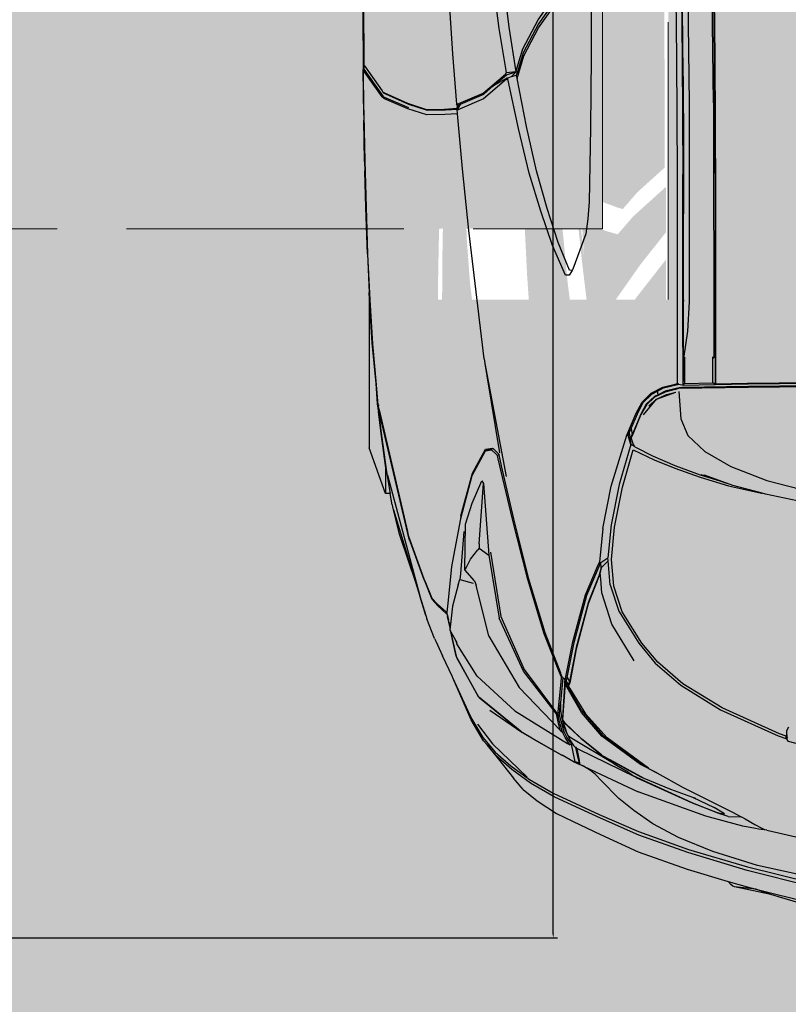
# Model space of a CAD drawing. Units: inches. Extents: x 1884 to 2398, y 474 to 1488.
# Tile 19 of 39: x 2275 to 2308, y 577 to 620. Entities that reach past the tile are written whole.
import ezdxf

# ---------------------------------------------------------------- set-up
doc = ezdxf.new("R2010")
doc.units = ezdxf.units.IN
doc.header["$MEASUREMENT"] = 0
doc.linetypes.add('ACAD_ISO02W100', pattern=[15, 12, -3])
doc.layers.get('0').update_dxf_attribs({"color": 250})
for name, color, linetype, lineweight in [('A-ANNO-DIMS', 2, 'Continuous', 18), ('A-FLOR-OVHD', 8, 'ACAD_ISO02W100', 18), ('C-VEHI', 8, 'Continuous', 18)]:
    doc.layers.add(name, color=color, linetype=linetype, lineweight=lineweight)
doc.layers.add('Edges', color=250, linetype='Continuous')
doc.layers.add('L-PVMT-PATT', color=9, linetype='Continuous', lineweight=13, true_color=0xc7c8ca)
doc.styles.get("Standard").update_dxf_attribs({"font": 'arial.ttf'})
doc.dimstyles.get("Standard").update_dxf_attribs({"dimtxt": 7, "dimasz": 0.18, "dimexe": 0.18, "dimexo": 0.0625, "dimgap": 0.09, "dimtad": 0, "dimtih": 1, "dimtoh": 1, "dimzin": 0, "dimdsep": 46, "dimlunit": 3, "dimtxsty": 'Standard', "dimcen": 0.09, "dimadec": 0, "dimazin": 0, "dimtfac": 1, "dimtofl": 0, "dimtmove": 0, "dimatfit": 3, "dimfxl": 1, "dimtolj": 1, "dimtzin": 0, "dimarcsym": 0})

# ---------------------------------------------------------------- blocks, each defined once
blk = doc.blocks.new('Nissan Qashqai pl')
at = {"layer": 'Edges'}
for p, q in [((11.0572, 11.4499), (11.056, 11.559)), ((11.0579, 11.4504), (11.0566, 11.5593)), ((11.0595, 11.5599), (11.0607, 11.4508)), ((11.0606, 11.5601), (11.0618, 11.4509)), ((11.6016, 11.5276), (11.5866, 11.4607)), ((11.5884, 11.4499), (11.6076, 11.5276)), ((11.6118, 11.5276), (11.5922, 11.4494)), ((11.6127, 11.4589), (11.6297, 11.5276)), ((11.164, 11.4711), (11.1776, 11.5231)), ((11.4503, 11.4945), (11.4568, 11.5197)), ((11.1877, 11.5111), (11.1791, 11.4696)), ((11.5481, 11.471), (11.5571, 11.511)), ((11.6277, 11.5063), (11.6224, 11.4874)), ((11.435, 11.4947), (11.439, 11.4927)), ((11.439, 11.4927), (11.4437, 11.4925)), ((11.4447, 11.4924), (11.4422, 11.4848)), ((11.4451, 11.4934), (11.4432, 11.4935)), ((11.4437, 11.4925), (11.4449, 11.4929)), ((11.4447, 11.4924), (11.4437, 11.4925)), ((11.4445, 11.4833), (11.4478, 11.493)), ((11.4449, 11.4929), (11.4447, 11.4924)), ((11.4462, 11.4924), (11.4447, 11.4924)), ((11.4449, 11.4929), (11.4461, 11.4934)), ((11.4451, 11.4934), (11.4449, 11.4929)), ((11.4461, 11.4934), (11.4451, 11.4934)), ((11.4479, 11.4933), (11.4461, 11.4934)), ((11.4479, 11.4933), (11.4462, 11.4924)), ((11.4478, 11.493), (11.4462, 11.4924)), ((11.4502, 11.4939), (11.4478, 11.493)), ((11.4503, 11.4945), (11.4479, 11.4932)), ((11.4479, 11.4932), (11.4479, 11.4933)), ((11.4502, 11.4939), (11.4503, 11.4945)), ((11.4422, 11.4848), (11.4138, 11.4219)), ((11.4159, 11.42), (11.4445, 11.4833)), ((11.6224, 11.4874), (11.6185, 11.4753)), ((11.1487, 11.4316), (11.164, 11.4711)), ((11.5481, 11.471), (11.5467, 11.462)), ((11.6185, 11.4753), (11.6101, 11.4356)), ((11.6174, 11.472), (11.6127, 11.4589)), ((11.6185, 11.4753), (11.6174, 11.472)), ((11.1781, 11.4659), (11.1694, 11.4337)), ((11.1699, 11.4289), (11.178, 11.4652)), ((11.178, 11.4652), (11.1781, 11.4659)), ((11.1791, 11.4696), (11.1781, 11.4659)), ((11.5416, 11.4578), (11.5455, 11.4648)), ((11.5455, 11.4648), (11.5472, 11.4684)), ((11.5467, 11.462), (11.5461, 11.4587)), ((11.5866, 11.4607), (11.5715, 11.4115)), ((11.0579, 11.4146), (11.0572, 11.4499)), ((11.0585, 11.4142), (11.0579, 11.4504)), ((11.0607, 11.4508), (11.0621, 11.3784)), ((11.0618, 11.4509), (11.0632, 11.3741)), ((11.5357, 11.4473), (11.5416, 11.4578)), ((11.5461, 11.4587), (11.5434, 11.4445)), ((11.5691, 11.385), (11.5884, 11.4499)), ((11.5922, 11.4494), (11.5726, 11.3842)), ((11.6042, 11.4286), (11.6103, 11.4492)), ((11.6127, 11.4589), (11.6101, 11.4356)), ((11.6103, 11.4492), (11.6127, 11.4589)), ((11.5283, 11.4332), (11.5334, 11.4428)), ((11.5326, 11.4397), (11.5333, 11.4423)), ((11.5331, 11.4285), (11.5335, 11.4431)), ((11.5333, 11.4423), (11.5334, 11.4428)), ((11.5334, 11.4428), (11.5335, 11.4431)), ((11.5335, 11.4431), (11.5357, 11.4473)), ((11.5434, 11.4445), (11.5386, 11.4254)), ((11.1323, 11.4027), (11.1487, 11.4316)), ((11.1605, 11.3977), (11.1699, 11.4289)), ((11.1694, 11.4337), (11.1668, 11.4265)), ((11.5202, 11.4171), (11.5283, 11.4332)), ((11.5331, 11.4285), (11.5292, 11.417)), ((11.5908, 11.3836), (11.6042, 11.4286)), ((11.6077, 11.4316), (11.6042, 11.4286)), ((11.6094, 11.4335), (11.6077, 11.4316)), ((11.6101, 11.4356), (11.6094, 11.4335)), ((11.1576, 11.3983), (11.1643, 11.4192)), ((11.1577, 11.3977), (11.1643, 11.4192)), ((11.1668, 11.4265), (11.1582, 11.4026)), ((11.1643, 11.4192), (11.1583, 11.4019)), ((11.1643, 11.4192), (11.1668, 11.4265)), ((11.4138, 11.4219), (11.3872, 11.3788)), ((11.3888, 11.3764), (11.4159, 11.42)), ((11.5013, 11.3791), (11.5202, 11.4171)), ((11.5292, 11.417), (11.5179, 11.389)), ((11.5301, 11.4244), (11.523, 11.4131)), ((11.5285, 11.4163), (11.5302, 11.4232)), ((11.5302, 11.4232), (11.5301, 11.4244)), ((11.5386, 11.4254), (11.5325, 11.4038)), ((10.6996, 11.4134), (10.5561, 11.4119)), ((10.5563, 11.4123), (10.6999, 11.4138)), ((10.7493, 11.4125), (10.6223, 11.4109)), ((10.7722, 11.4138), (10.6996, 11.4134)), ((10.6999, 11.4138), (10.7722, 11.4142)), ((10.7493, 11.4125), (11.0294, 11.4126)), ((10.7722, 11.4142), (10.7889, 11.4143)), ((10.7722, 11.4142), (10.7722, 11.4138)), ((10.7889, 11.4139), (10.7722, 11.4138)), ((10.7889, 11.4139), (10.7889, 11.4143)), ((10.7889, 11.4143), (10.7923, 11.4143)), ((10.7923, 11.4139), (10.7889, 11.4139)), ((10.7923, 11.4139), (10.7923, 11.4143)), ((10.7923, 11.4143), (10.7933, 11.4143)), ((10.7933, 11.4139), (10.7923, 11.4139)), ((10.7933, 11.4143), (10.827, 11.4145)), ((10.7933, 11.4139), (10.7933, 11.4143)), ((10.8267, 11.4141), (10.7933, 11.4139)), ((10.8267, 11.4141), (11.0585, 11.4142)), ((10.827, 11.4145), (11.0579, 11.4146)), ((11.0294, 11.4118), (11.0281, 11.4118)), ((11.0294, 11.4125), (11.0294, 11.4126)), ((11.0295, 11.4116), (11.0294, 11.4118)), ((11.0568, 11.4118), (11.0294, 11.4118)), ((11.0585, 11.4142), (11.0568, 11.4118)), ((11.0574, 11.3804), (11.0568, 11.4118)), ((11.0585, 11.4142), (11.0579, 11.4146)), ((11.0592, 11.3789), (11.0585, 11.4142)), ((11.5118, 11.3894), (11.523, 11.4131)), ((11.5179, 11.389), (11.5285, 11.4163)), ((11.5715, 11.4115), (11.5562, 11.3741)), ((11.1148, 11.3843), (11.1323, 11.4027)), ((11.1475, 11.37), (11.1577, 11.3977)), ((11.1505, 11.37), (11.1605, 11.3977)), ((11.5325, 11.4038), (11.5057, 11.3296)), ((10.6237, 11.3839), (10.7502, 11.3855)), ((10.7502, 11.3855), (10.968, 11.3857)), ((10.968, 11.3857), (11, 11.3837)), ((11.0962, 11.3766), (11.1148, 11.3843)), ((11.5179, 11.389), (11.488, 11.3234)), ((11.49, 11.3275), (11.5179, 11.389)), ((11.5028, 11.365), (11.5118, 11.3894)), ((11.5118, 11.3894), (11.513, 11.3927)), ((11.5496, 11.33), (11.5691, 11.385)), ((11.5726, 11.3842), (11.5535, 11.3303)), ((10.5566, 11.3765), (10.7, 11.378)), ((10.6649, 11.3783), (10.5576, 11.3766)), ((10.6649, 11.3783), (10.5866, 11.3772)), ((10.6908, 11.3785), (10.6649, 11.3783)), ((10.6649, 11.3783), (10.6772, 11.3784)), ((10.6966, 11.3787), (10.6772, 11.3784)), ((10.6772, 11.3784), (10.6908, 11.3785)), ((10.6991, 11.3786), (10.6908, 11.3785)), ((10.7144, 11.3788), (10.6966, 11.3787)), ((10.6999, 11.3786), (10.6991, 11.3786)), ((10.6999, 11.3786), (10.7808, 11.3793)), ((10.7144, 11.3788), (10.6999, 11.3786)), ((10.7, 11.378), (10.8279, 11.3787)), ((10.7239, 11.3789), (10.7144, 11.3788)), ((10.7248, 11.3789), (10.7239, 11.3789)), ((10.7808, 11.3793), (10.7248, 11.3789)), ((10.7808, 11.3793), (10.8711, 11.3796)), ((10.9431, 11.3796), (10.8279, 11.3787)), ((10.8279, 11.3787), (11.0552, 11.3789)), ((10.9614, 11.3788), (10.8279, 11.3787)), ((10.896, 11.3796), (10.8711, 11.3796)), ((10.9097, 11.3796), (10.896, 11.3796)), ((10.9431, 11.3796), (10.9097, 11.3796)), ((10.9478, 11.3796), (10.9431, 11.3796)), ((10.9491, 11.3796), (10.9478, 11.3796)), ((10.9668, 11.3796), (10.9491, 11.3796)), ((10.9614, 11.3788), (10.9668, 11.3796)), ((10.9711, 11.3788), (10.9614, 11.3788)), ((10.9668, 11.3796), (10.967, 11.3796)), ((10.9765, 11.3796), (10.967, 11.3796)), ((10.9765, 11.3796), (10.9711, 11.3788)), ((10.9766, 11.3788), (10.9711, 11.3788)), ((10.9765, 11.3796), (10.9766, 11.3788)), ((10.9825, 11.3796), (10.9765, 11.3796)), ((11.0592, 11.3789), (10.9766, 11.3788)), ((11.0301, 11.3796), (10.9825, 11.3796)), ((11, 11.3837), (11.0301, 11.3796)), ((11.0287, 11.3804), (11.0301, 11.3804)), ((11.0301, 11.3803), (11.0292, 11.3802)), ((11.03, 11.3822), (11.03, 11.3824)), ((11.0301, 11.3803), (11.0301, 11.3804)), ((11.0301, 11.3804), (11.0554, 11.3804)), ((11.0554, 11.3804), (11.0301, 11.3803)), ((11.0301, 11.3796), (11.0301, 11.3803)), ((11.0554, 11.3804), (11.0574, 11.3804)), ((11.0592, 11.3789), (11.0574, 11.3804)), ((11.0582, 11.3742), (11.0575, 11.3728)), ((11.0582, 11.3742), (11.0592, 11.3789)), ((11.0624, 11.3576), (11.0582, 11.3742)), ((11.0621, 11.3784), (11.0622, 11.3745)), ((11.0622, 11.3745), (11.063, 11.3714)), ((11.0632, 11.3741), (11.0641, 11.3708)), ((11.0662, 11.3744), (11.0962, 11.3766)), ((11.3872, 11.3788), (11.3635, 11.3513)), ((11.3645, 11.3484), (11.3888, 11.3764)), ((11.4852, 11.3502), (11.5013, 11.3791)), ((11.5562, 11.3741), (11.541, 11.3459)), ((11.5716, 11.3297), (11.5908, 11.3836)), ((10.7004, 11.372), (10.5572, 11.3704)), ((10.8279, 11.3727), (10.7004, 11.372)), ((11.0544, 11.3728), (10.8279, 11.3727)), ((11.0575, 11.3728), (11.0544, 11.3728)), ((11.0581, 11.3704), (11.0575, 11.3728)), ((11.0614, 11.3569), (11.0581, 11.3704)), ((11.063, 11.3714), (11.0659, 11.3594)), ((11.0641, 11.3708), (11.0669, 11.3592)), ((11.0696, 11.3606), (11.0671, 11.3711)), ((11.0747, 11.3498), (11.0671, 11.3711)), ((11.1369, 11.3455), (11.1475, 11.37)), ((11.1412, 11.3473), (11.1505, 11.37)), ((11.4909, 11.3357), (11.5028, 11.365)), ((11.0682, 11.3438), (11.0614, 11.3569)), ((11.0658, 11.3509), (11.0624, 11.3576)), ((11.0659, 11.3594), (11.0698, 11.3516)), ((11.0669, 11.3592), (11.0727, 11.3475)), ((11.0747, 11.3498), (11.0696, 11.3606)), ((11.0698, 11.3516), (11.0658, 11.3509)), ((11.0692, 11.3445), (11.0658, 11.3509)), ((11.0779, 11.3339), (11.0682, 11.3438)), ((11.0787, 11.3349), (11.0692, 11.3445)), ((11.0698, 11.3516), (11.0718, 11.3475)), ((11.0718, 11.3475), (11.0802, 11.3384)), ((11.0727, 11.3475), (11.0809, 11.3386)), ((11.0821, 11.3412), (11.0747, 11.3498)), ((11.092, 11.3355), (11.0747, 11.3498)), ((11.1277, 11.3275), (11.1369, 11.3455)), ((11.1302, 11.3242), (11.1412, 11.3473)), ((11.3635, 11.3513), (11.3425, 11.3336)), ((11.3428, 11.3303), (11.3645, 11.3484)), ((11.48, 11.341), (11.4467, 11.2954)), ((11.4852, 11.3502), (11.4758, 11.3323)), ((11.4788, 11.339), (11.48, 11.341)), ((11.48, 11.341), (11.4801, 11.3411)), ((11.4801, 11.3411), (11.4852, 11.3502)), ((11.541, 11.3459), (11.5265, 11.3247)), ((11.0902, 11.3275), (11.0779, 11.3339)), ((11.0908, 11.3288), (11.0787, 11.3349)), ((11.0802, 11.3384), (11.0912, 11.3325)), ((11.0809, 11.3386), (11.0917, 11.3327)), ((11.0912, 11.3325), (11.1138, 11.3229)), ((11.0917, 11.3327), (11.1149, 11.323)), ((11.3076, 11.3083), (11.3428, 11.3303)), ((11.3425, 11.3336), (11.3082, 11.3121)), ((11.4433, 11.2899), (11.4745, 11.3325)), ((11.4758, 11.3323), (11.4447, 11.2897)), ((11.4633, 11.2847), (11.4897, 11.3334)), ((11.4704, 11.2984), (11.4909, 11.3357)), ((11.4704, 11.2984), (11.4897, 11.3334)), ((11.4788, 11.339), (11.4745, 11.3325)), ((11.4897, 11.3334), (11.4909, 11.3357)), ((11.5535, 11.3303), (11.5349, 11.2883)), ((11.1144, 11.3171), (11.0902, 11.3275)), ((11.107, 11.3218), (11.0908, 11.3288)), ((11.107, 11.3218), (11.1138, 11.3229)), ((11.1116, 11.3198), (11.107, 11.3218)), ((11.1116, 11.3198), (11.1244, 11.3215)), ((11.1147, 11.3185), (11.1116, 11.3198)), ((11.1138, 11.3229), (11.1139, 11.3228)), ((11.1139, 11.3228), (11.1164, 11.3217)), ((11.1244, 11.3215), (11.1147, 11.3185)), ((11.1149, 11.323), (11.1172, 11.322)), ((11.1164, 11.3217), (11.1172, 11.322)), ((11.1174, 11.3219), (11.1164, 11.3217)), ((11.1172, 11.322), (11.1174, 11.3219)), ((11.1174, 11.3219), (11.12, 11.3227)), ((11.12, 11.3227), (11.1246, 11.3243)), ((11.126, 11.3248), (11.1244, 11.3215)), ((11.1244, 11.3215), (11.1259, 11.3248)), ((11.1244, 11.3215), (11.1684, 11.3087)), ((11.1246, 11.3243), (11.1259, 11.3248)), ((11.1247, 11.3244), (11.126, 11.3249)), ((11.1248, 11.3247), (11.126, 11.3249)), ((11.126, 11.3249), (11.1251, 11.3253)), ((11.1259, 11.3248), (11.126, 11.3249)), ((11.1259, 11.3248), (11.126, 11.3248)), ((11.126, 11.3249), (11.1263, 11.3255)), ((11.126, 11.3248), (11.1264, 11.325)), ((11.126, 11.3249), (11.1261, 11.3249)), ((11.1261, 11.3249), (11.126, 11.3248)), ((11.1263, 11.3254), (11.1261, 11.3249)), ((11.1261, 11.3249), (11.1264, 11.325)), ((11.1264, 11.325), (11.1277, 11.3275)), ((11.1712, 11.3124), (11.1302, 11.3242)), ((11.3619, 11.3254), (11.3218, 11.3008)), ((11.4588, 11.2635), (11.4895, 11.3264)), ((11.4813, 11.2773), (11.5057, 11.3296)), ((11.488, 11.3234), (11.4828, 11.3165)), ((11.4898, 11.3269), (11.4895, 11.3264)), ((11.4898, 11.3269), (11.49, 11.3275)), ((11.5265, 11.3247), (11.5131, 11.3085)), ((11.5306, 11.2869), (11.5496, 11.33)), ((11.5527, 11.2882), (11.5716, 11.3297)), ((11.1702, 11.2998), (11.1144, 11.3171)), ((11.1684, 11.3087), (11.2127, 11.2998)), ((11.2152, 11.3038), (11.1712, 11.3124)), ((11.3082, 11.3121), (11.28, 11.3028)), ((11.475, 11.3032), (11.4828, 11.3165)), ((11.5131, 11.3085), (11.4933, 11.2891)), ((11.2166, 11.2908), (11.1702, 11.2998)), ((11.2127, 11.2998), (11.2488, 11.2962)), ((11.2509, 11.3003), (11.2152, 11.3038)), ((11.28, 11.3028), (11.2509, 11.3003)), ((11.2785, 11.2987), (11.2524, 11.2965)), ((11.2785, 11.2987), (11.3076, 11.3083)), ((11.3218, 11.3008), (11.2874, 11.2897)), ((11.475, 11.3032), (11.4462, 11.2548)), ((11.4675, 11.2931), (11.4703, 11.2982)), ((11.4703, 11.2982), (11.4704, 11.2984)), ((11.2166, 11.2908), (11.2538, 11.2871)), ((11.2524, 11.2965), (11.2488, 11.2962)), ((11.2541, 11.2885), (11.2488, 11.2962)), ((11.2524, 11.2965), (11.2599, 11.2889)), ((11.2586, 11.285), (11.2538, 11.2871)), ((11.2599, 11.2889), (11.2541, 11.2885)), ((11.29, 11.2731), (11.2541, 11.2885)), ((11.2599, 11.2889), (11.26, 11.2889)), ((11.26, 11.2889), (11.265, 11.2879)), ((11.26, 11.2889), (11.2677, 11.2867)), ((11.2724, 11.2885), (11.265, 11.2879)), ((11.265, 11.2879), (11.2705, 11.2862)), ((11.2874, 11.2897), (11.2724, 11.2885)), ((11.4171, 11.2676), (11.4433, 11.2899)), ((11.4447, 11.2897), (11.4187, 11.2673)), ((11.4203, 11.2717), (11.4467, 11.2954)), ((11.4469, 11.2668), (11.4659, 11.2902)), ((11.4654, 11.2893), (11.4479, 11.2676)), ((11.4654, 11.2893), (11.4659, 11.2902)), ((11.4659, 11.2902), (11.4674, 11.2929)), ((11.4675, 11.2931), (11.4674, 11.2929)), ((11.4933, 11.2891), (11.4869, 11.2826)), ((11.5165, 11.256), (11.5306, 11.2869)), ((11.5349, 11.2883), (11.5206, 11.2572)), ((11.5384, 11.2583), (11.5527, 11.2882)), ((10.5892, 11.2783), (10.6988, 11.2779)), ((10.6988, 11.2779), (10.7769, 11.2774)), ((10.7769, 11.2774), (10.858, 11.2759)), ((11.2895, 11.2718), (11.2586, 11.285)), ((11.2677, 11.2867), (11.2678, 11.2866)), ((11.2678, 11.2866), (11.2972, 11.2749)), ((11.2705, 11.2862), (11.2993, 11.2747)), ((11.4771, 11.2681), (11.4813, 11.2773)), ((11.4826, 11.2772), (11.4778, 11.2695)), ((11.4813, 11.2773), (11.4822, 11.2786)), ((11.4869, 11.2826), (11.4826, 11.2772)), ((10.858, 11.2759), (10.8766, 11.2745)), ((10.8766, 11.2745), (10.8932, 11.2722)), ((10.8932, 11.2722), (10.932, 11.258)), ((11.3411, 11.2579), (11.2895, 11.2718)), ((11.3419, 11.2592), (11.29, 11.2731)), ((11.2972, 11.2749), (11.3474, 11.2614)), ((11.2993, 11.2747), (11.3493, 11.2614)), ((11.4171, 11.2676), (11.3851, 11.2491)), ((11.4187, 11.2673), (11.3914, 11.2516)), ((11.3923, 11.2547), (11.4203, 11.2717)), ((11.4296, 11.2488), (11.4469, 11.2668)), ((11.4479, 11.2676), (11.4303, 11.2485)), ((11.4778, 11.2695), (11.4759, 11.2652)), ((11.4771, 11.2681), (11.4759, 11.2652)), ((10.932, 11.258), (10.9335, 11.257)), ((10.9335, 11.257), (10.933, 11.2541)), ((10.9335, 11.257), (10.9386, 11.2537)), ((11.3795, 11.2503), (11.3411, 11.2579)), ((11.3804, 11.2515), (11.3419, 11.2592)), ((11.3474, 11.2614), (11.3848, 11.2543)), ((11.3493, 11.2614), (11.3863, 11.2544)), ((11.3863, 11.2544), (11.3895, 11.253)), ((11.3895, 11.253), (11.3923, 11.2547)), ((11.4442, 11.2522), (11.4497, 11.2552)), ((11.4462, 11.2548), (11.4442, 11.2522)), ((11.4512, 11.2549), (11.4457, 11.2513)), ((11.4497, 11.2552), (11.4498, 11.2553)), ((11.4498, 11.2553), (11.4549, 11.2587)), ((11.4498, 11.2553), (11.4535, 11.2565)), ((11.4512, 11.2549), (11.4535, 11.2565)), ((11.4539, 11.2545), (11.452, 11.2532)), ((11.4529, 11.252), (11.4542, 11.2547)), ((11.4532, 11.256), (11.4535, 11.2565)), ((11.4728, 11.2604), (11.4535, 11.2565)), ((11.4535, 11.2565), (11.4542, 11.2547)), ((11.4542, 11.2547), (11.4539, 11.2545)), ((11.4549, 11.2587), (11.4568, 11.2605)), ((11.4564, 11.2609), (11.4567, 11.2609)), ((11.4565, 11.261), (11.4569, 11.2611)), ((11.4568, 11.2605), (11.4571, 11.2609)), ((11.4571, 11.2609), (11.4573, 11.2612)), ((11.4704, 11.2639), (11.4573, 11.2612)), ((11.4573, 11.2612), (11.4578, 11.262)), ((11.4574, 11.2619), (11.4573, 11.2619)), ((11.4573, 11.2619), (11.4573, 11.2619)), ((11.4574, 11.2619), (11.4576, 11.2619)), ((11.4578, 11.262), (11.4588, 11.2635)), ((11.4578, 11.262), (11.4605, 11.2625)), ((11.4605, 11.2625), (11.4713, 11.2647)), ((11.4605, 11.2625), (11.4605, 11.2625)), ((11.4732, 11.2592), (11.4658, 11.2461)), ((11.4704, 11.2639), (11.4742, 11.2645)), ((11.4713, 11.2647), (11.4744, 11.265)), ((11.472, 11.2571), (11.4718, 11.2568)), ((11.4727, 11.2601), (11.4728, 11.2603)), ((11.4746, 11.2646), (11.4728, 11.2604)), ((11.4742, 11.2645), (11.4728, 11.2604)), ((11.4728, 11.2603), (11.4732, 11.261)), ((11.4728, 11.2604), (11.4728, 11.2603)), ((11.4728, 11.2603), (11.4732, 11.2592)), ((11.4758, 11.2651), (11.4732, 11.2592)), ((11.4742, 11.2645), (11.4745, 11.2645)), ((11.4744, 11.265), (11.4743, 11.2647)), ((11.4744, 11.265), (11.4745, 11.265)), ((11.4745, 11.2648), (11.4745, 11.265)), ((11.4745, 11.265), (11.4748, 11.265)), ((11.4746, 11.2646), (11.4745, 11.2645)), ((11.4758, 11.2651), (11.4746, 11.2646)), ((11.4748, 11.265), (11.4747, 11.2648)), ((11.4748, 11.265), (11.4758, 11.2651)), ((11.4759, 11.2652), (11.4758, 11.2651)), ((11.5074, 11.2362), (11.5165, 11.256)), ((11.5206, 11.2572), (11.5113, 11.2372)), ((11.5295, 11.24), (11.5384, 11.2583)), ((10.6583, 11.2197), (10.6215, 11.2456)), ((10.6261, 11.2458), (10.6627, 11.22)), ((10.6671, 11.2203), (10.6306, 11.2459)), ((10.933, 11.2541), (10.9026, 11.2417)), ((10.9384, 11.2497), (10.9059, 11.2355)), ((10.9386, 11.2537), (10.9384, 11.2497)), ((11.3311, 11.227), (11.3751, 11.2443)), ((11.38, 11.2453), (11.3747, 11.2431)), ((11.3751, 11.2443), (11.3752, 11.2444)), ((11.3751, 11.2443), (11.3762, 11.2443)), ((11.3792, 11.2459), (11.3752, 11.2444)), ((11.3763, 11.2444), (11.3752, 11.2444)), ((11.3792, 11.2459), (11.3804, 11.2469)), ((11.3793, 11.2463), (11.3792, 11.2459)), ((11.3834, 11.2495), (11.3795, 11.2503)), ((11.3853, 11.2449), (11.38, 11.2453)), ((11.3804, 11.2515), (11.3848, 11.2543)), ((11.3841, 11.2508), (11.3804, 11.2515)), ((11.3804, 11.2469), (11.3827, 11.2489)), ((11.3804, 11.2469), (11.4082, 11.2444)), ((11.3813, 11.2485), (11.3817, 11.2488)), ((11.3827, 11.2489), (11.3834, 11.2495)), ((11.3829, 11.249), (11.388, 11.2532)), ((11.3845, 11.2498), (11.3829, 11.249)), ((11.3829, 11.249), (11.3849, 11.2491)), ((11.3829, 11.249), (11.3846, 11.2488)), ((11.3841, 11.2508), (11.3834, 11.2495)), ((11.3846, 11.2489), (11.385, 11.2491)), ((11.3849, 11.2491), (11.3846, 11.2489)), ((11.3846, 11.2488), (11.3846, 11.2489)), ((11.3846, 11.2488), (11.3893, 11.2486)), ((11.3848, 11.2543), (11.388, 11.2532)), ((11.3882, 11.2519), (11.3849, 11.2491)), ((11.385, 11.2491), (11.3851, 11.2491)), ((11.3851, 11.2491), (11.3867, 11.2492)), ((11.4212, 11.2412), (11.3853, 11.2449)), ((11.3881, 11.2519), (11.3861, 11.2508)), ((11.3914, 11.2516), (11.3867, 11.2492)), ((11.3867, 11.2492), (11.3915, 11.2491)), ((11.3886, 11.2522), (11.3882, 11.2519)), ((11.3886, 11.2522), (11.3882, 11.252)), ((11.3906, 11.2534), (11.3886, 11.2522)), ((11.3895, 11.253), (11.3886, 11.2522)), ((11.3893, 11.2486), (11.4248, 11.2465)), ((11.3915, 11.2491), (11.4266, 11.2465)), ((11.3915, 11.1988), (11.4381, 11.244)), ((11.4164, 11.2444), (11.4082, 11.2444)), ((11.409, 11.2443), (11.4082, 11.2444)), ((11.409, 11.2443), (11.4163, 11.2443)), ((11.4152, 11.2437), (11.409, 11.2443)), ((11.4163, 11.2443), (11.4152, 11.2437)), ((11.4215, 11.2431), (11.4152, 11.2437)), ((11.4164, 11.2444), (11.4163, 11.2443)), ((11.4169, 11.2446), (11.4164, 11.2444)), ((11.4252, 11.2462), (11.4169, 11.2446)), ((11.417, 11.1942), (11.4529, 11.252)), ((11.4315, 11.244), (11.4229, 11.2416)), ((11.44, 11.2482), (11.423, 11.2435)), ((11.4248, 11.2465), (11.4266, 11.2465)), ((11.4266, 11.2465), (11.4252, 11.2462)), ((11.4266, 11.2465), (11.4268, 11.2465)), ((11.4268, 11.2465), (11.4296, 11.2488)), ((11.4268, 11.2465), (11.4278, 11.2465)), ((11.4303, 11.2485), (11.4278, 11.2465)), ((11.4278, 11.2465), (11.43, 11.2472)), ((11.4381, 11.244), (11.4292, 11.2418)), ((11.43, 11.2472), (11.4361, 11.2494)), ((11.4337, 11.248), (11.43, 11.2472)), ((11.4403, 11.2464), (11.4315, 11.244)), ((11.4397, 11.2505), (11.4337, 11.248)), ((11.4361, 11.2494), (11.4406, 11.251)), ((11.4381, 11.244), (11.4403, 11.2464)), ((11.4406, 11.251), (11.4397, 11.2505)), ((11.4457, 11.2513), (11.44, 11.2482)), ((11.4403, 11.2464), (11.44, 11.2482)), ((11.4462, 11.2495), (11.4403, 11.2464)), ((11.4406, 11.251), (11.4442, 11.2522)), ((11.4411, 11.2028), (11.4656, 11.2458)), ((11.452, 11.2532), (11.4462, 11.2495)), ((11.447, 11.2127), (11.4656, 11.2458)), ((11.4656, 11.2458), (11.4658, 11.2461)), ((10.9026, 11.2417), (10.8653, 11.2297)), ((10.9059, 11.2355), (10.8682, 11.2226)), ((11.3747, 11.2431), (11.3323, 11.2264)), ((11.3715, 11.2043), (11.4177, 11.2389)), ((11.4203, 11.2398), (11.3733, 11.2037)), ((11.4177, 11.2389), (11.4193, 11.24)), ((11.4192, 11.2397), (11.4194, 11.24)), ((11.4193, 11.24), (11.4196, 11.2402)), ((11.4194, 11.24), (11.4193, 11.24)), ((11.4194, 11.24), (11.4196, 11.2402)), ((11.4196, 11.2399), (11.4194, 11.24)), ((11.4196, 11.2402), (11.4201, 11.2405)), ((11.4198, 11.2401), (11.4201, 11.2405)), ((11.4201, 11.2405), (11.4212, 11.2412)), ((11.4292, 11.2418), (11.4203, 11.2398)), ((11.4229, 11.2416), (11.4203, 11.2398)), ((11.4212, 11.2412), (11.4215, 11.2431)), ((11.4218, 11.2413), (11.4212, 11.2412)), ((11.423, 11.2435), (11.4215, 11.2431)), ((11.4229, 11.2416), (11.4218, 11.2413)), ((11.4222, 11.2413), (11.4218, 11.2413)), ((11.423, 11.2435), (11.4229, 11.2416)), ((11.4924, 11.2103), (11.5074, 11.2362)), ((11.5113, 11.2372), (11.4963, 11.2114)), ((11.5158, 11.2186), (11.5295, 11.24)), ((10.8653, 11.2297), (10.8239, 11.2181)), ((10.8682, 11.2226), (10.8264, 11.21)), ((11.272, 11.2092), (11.3311, 11.227)), ((11.3323, 11.2264), (11.2728, 11.2084)), ((10.69, 11.2028), (10.6583, 11.2197)), ((10.6627, 11.22), (10.6943, 11.2032)), ((10.6976, 11.2041), (10.6671, 11.2203)), ((10.8239, 11.2181), (10.7754, 11.2071)), ((11.447, 11.2127), (11.4411, 11.2028)), ((11.4963, 11.2114), (11.4815, 11.191)), ((11.5033, 11.2034), (11.5158, 11.2186)), ((10.7155, 11.1952), (10.69, 11.2028)), ((10.6943, 11.2032), (10.7155, 11.1969)), ((10.7228, 11.1965), (10.6976, 11.2041)), ((10.7754, 11.2071), (10.7228, 11.1965)), ((10.8264, 11.21), (10.7776, 11.1982)), ((11.2063, 11.1926), (11.272, 11.2092)), ((11.2728, 11.2084), (11.2066, 11.1914)), ((11.3132, 11.1789), (11.3715, 11.2043)), ((11.3733, 11.2037), (11.3153, 11.1769)), ((11.4405, 11.2018), (11.4014, 11.1541)), ((11.4022, 11.1548), (11.4405, 11.2018)), ((11.4163, 11.1666), (11.4405, 11.2018)), ((11.4408, 11.2022), (11.4405, 11.2018)), ((11.4411, 11.2028), (11.4408, 11.2022)), ((11.4411, 11.2028), (11.4411, 11.2028)), ((11.4531, 11.1697), (11.4897, 11.2077)), ((11.4774, 11.1898), (11.4924, 11.2103)), ((11.5033, 11.2034), (11.4936, 11.195)), ((10.6664, 11.1875), (10.7155, 11.1952)), ((10.7155, 11.1957), (10.7155, 11.1969)), ((10.7155, 11.1969), (10.7192, 11.1957)), ((10.7209, 11.1902), (10.7155, 11.1957)), ((10.7155, 11.1952), (10.7155, 11.1957)), ((10.7186, 11.1848), (10.7155, 11.1952)), ((10.7155, 11.1952), (10.7165, 11.1851)), ((10.7192, 11.1957), (10.7228, 11.1965)), ((10.7192, 11.1957), (10.7209, 11.1902)), ((10.7209, 11.1902), (10.7221, 11.1861)), ((10.7776, 11.1982), (10.7247, 11.1867)), ((11.2066, 11.1914), (11.1401, 11.1759)), ((11.148, 11.1791), (11.2063, 11.1926)), ((11.335, 11.1656), (11.3915, 11.1988)), ((11.379, 11.1527), (11.417, 11.1942)), ((11.4543, 11.1636), (11.4908, 11.1928)), ((11.4624, 11.1725), (11.4774, 11.1898)), ((11.4815, 11.191), (11.4662, 11.1736)), ((11.4936, 11.195), (11.4908, 11.1928)), ((10.6144, 11.1813), (10.6664, 11.1875)), ((10.7137, 11.1846), (10.6678, 11.177)), ((10.7165, 11.1851), (10.7137, 11.1846)), ((10.7177, 11.1838), (10.7165, 11.1851)), ((10.7387, 11.1593), (10.7177, 11.1838)), ((10.7312, 11.1701), (10.7186, 11.1848)), ((10.7221, 11.1861), (10.7222, 11.1859)), ((10.7222, 11.186), (10.7221, 11.1861)), ((10.7247, 11.1867), (10.7222, 11.186)), ((10.7222, 11.186), (10.7222, 11.1859)), ((10.7222, 11.1859), (10.7232, 11.1848)), ((10.7222, 11.1859), (10.7224, 11.1855)), ((10.7224, 11.1855), (10.7312, 11.1701)), ((10.7232, 11.1848), (10.7228, 11.1859)), ((10.7232, 11.1848), (10.7449, 11.1598)), ((10.7257, 11.1853), (10.7256, 11.1854)), ((11.0357, 11.1613), (11.1598, 11.1847)), ((11.1358, 11.1765), (11.148, 11.1791)), ((11.2428, 11.1673), (11.3132, 11.1789)), ((10.6678, 11.177), (10.6152, 11.1702)), ((10.7397, 11.1602), (10.7312, 11.1701)), ((11.0492, 11.1635), (11.1336, 11.1772)), ((11.1285, 11.1697), (11.1293, 11.1705)), ((11.1298, 11.1618), (11.1285, 11.1697)), ((11.1293, 11.1705), (11.1353, 11.1764)), ((11.1293, 11.1705), (11.1306, 11.163)), ((11.1347, 11.1731), (11.1306, 11.169)), ((11.1306, 11.169), (11.1319, 11.1614)), ((11.1366, 11.175), (11.1347, 11.1731)), ((11.1353, 11.1764), (11.1358, 11.1765)), ((11.1358, 11.1765), (11.1366, 11.175)), ((11.1401, 11.1759), (11.1366, 11.175)), ((11.2459, 11.1656), (11.3153, 11.1769)), ((11.4314, 11.1531), (11.4531, 11.1697)), ((11.4464, 11.1588), (11.4624, 11.1725)), ((11.4662, 11.1736), (11.4543, 11.1636)), ((10.7501, 11.1327), (10.7387, 11.1593)), ((10.7507, 11.1344), (10.7397, 11.1602)), ((10.7449, 11.1598), (10.7563, 11.1333)), ((11.0304, 11.1603), (10.8896, 11.1434)), ((11.0304, 11.1603), (11.0357, 11.1613)), ((11.0357, 11.1613), (11.0491, 11.1635)), ((11.0492, 11.1635), (11.0491, 11.1635)), ((11.156, 11.1476), (11.1298, 11.1618)), ((11.1319, 11.1614), (11.1306, 11.163)), ((11.1319, 11.1614), (11.1365, 11.159)), ((11.1365, 11.159), (11.1589, 11.147)), ((11.1644, 11.1579), (11.1672, 11.1598)), ((11.189, 11.1473), (11.1644, 11.1579)), ((11.1672, 11.1598), (11.2459, 11.1656)), ((11.2337, 11.155), (11.1672, 11.1598)), ((11.2382, 11.1549), (11.2459, 11.1656)), ((11.335, 11.1656), (11.2791, 11.1515)), ((11.4243, 11.1459), (11.4464, 11.1588)), ((11.4498, 11.1598), (11.4267, 11.1463)), ((11.4543, 11.1636), (11.4498, 11.1598)), ((11.2029, 11.1349), (11.156, 11.1476)), ((11.1589, 11.147), (11.2062, 11.1344)), ((11.2121, 11.1399), (11.189, 11.1473)), ((11.2337, 11.155), (11.2382, 11.1549)), ((11.2382, 11.1549), (11.2401, 11.1534)), ((11.2505, 11.1455), (11.2401, 11.1534)), ((11.2743, 11.1499), (11.2622, 11.139)), ((11.2729, 11.1338), (11.2766, 11.1485)), ((11.2743, 11.1499), (11.2791, 11.1515)), ((11.379, 11.1527), (11.3434, 11.1303)), ((11.4014, 11.1541), (11.3571, 11.1296)), ((11.3583, 11.13), (11.4014, 11.1541)), ((11.4267, 11.1463), (11.3807, 11.1259)), ((11.4022, 11.1548), (11.4014, 11.1541)), ((10.8218, 11.1365), (10.7615, 11.1311)), ((10.8896, 11.1434), (10.8218, 11.1365)), ((11.2622, 11.139), (11.2121, 11.1399)), ((11.2199, 11.1382), (11.2666, 11.1345)), ((11.2601, 11.1405), (11.2505, 11.1455)), ((11.2622, 11.139), (11.2601, 11.1405)), ((11.4228, 11.1453), (11.3807, 11.1259)), ((11.4228, 11.1453), (11.4243, 11.1459)), ((10.6318, 11.1213), (10.6955, 11.1257)), ((10.6955, 11.1257), (10.7509, 11.1302)), ((10.7507, 11.1309), (10.7501, 11.1327)), ((10.7511, 11.1335), (10.7507, 11.1344)), ((10.7507, 11.1344), (10.7524, 11.1335)), ((10.751, 11.131), (10.7507, 11.1309)), ((10.7509, 11.1302), (10.7507, 11.1309)), ((10.7522, 11.1311), (10.7509, 11.1302)), ((10.7516, 11.131), (10.7509, 11.1302)), ((10.7519, 11.1314), (10.7511, 11.1335)), ((10.7519, 11.1314), (10.7516, 11.131)), ((10.7522, 11.1311), (10.7516, 11.131)), ((10.7526, 11.1318), (10.7519, 11.1314)), ((10.7553, 11.1307), (10.7522, 11.1311)), ((10.7524, 11.1335), (10.7526, 11.1318)), ((10.7524, 11.1335), (10.7556, 11.1319)), ((10.7532, 11.1321), (10.7526, 11.1318)), ((10.7526, 11.1318), (10.7526, 11.1314)), ((10.7556, 11.1319), (10.7532, 11.1321)), ((10.7563, 11.1169), (10.7553, 11.1307)), ((10.7556, 11.1319), (10.7561, 11.1317)), ((10.7563, 11.1319), (10.7561, 11.1319)), ((10.7563, 11.1315), (10.7561, 11.1317)), ((10.7561, 11.1317), (10.7563, 11.1317)), ((10.7563, 11.1333), (10.7569, 11.1317)), ((10.7563, 11.1317), (10.7563, 11.1319)), ((10.7563, 11.1317), (10.7569, 11.1317)), ((10.7569, 11.1316), (10.7563, 11.1317)), ((10.7563, 11.1315), (10.7563, 11.1317)), ((10.7572, 11.1178), (10.7563, 11.1315)), ((10.7573, 11.1307), (10.7563, 11.1315)), ((10.7569, 11.1317), (10.7569, 11.1316)), ((10.7569, 11.1316), (10.7573, 11.1307)), ((10.7604, 11.131), (10.7573, 11.1307)), ((10.7615, 11.1311), (10.7604, 11.131)), ((10.7615, 11.1311), (10.7623, 11.1173)), ((11.2029, 11.1349), (11.2029, 11.1349)), ((11.2029, 11.1349), (11.2062, 11.1344)), ((11.2062, 11.1344), (11.2583, 11.1246)), ((11.2666, 11.1345), (11.2729, 11.1338)), ((11.2787, 11.1318), (11.2729, 11.1338)), ((11.2787, 11.1318), (11.3022, 11.1256)), ((11.3022, 11.1256), (11.3252, 11.1229)), ((11.3296, 11.1235), (11.3571, 11.1296)), ((11.3571, 11.1296), (11.3302, 11.1238)), ((11.3302, 11.1238), (11.3394, 11.129)), ((11.3394, 11.129), (11.342, 11.1305)), ((11.3394, 11.129), (11.3434, 11.1303)), ((11.3796, 11.1255), (11.3566, 11.1148)), ((11.3571, 11.1296), (11.3583, 11.13)), ((11.3807, 11.1259), (11.3796, 11.1255)), ((10.7565, 11.0969), (10.7563, 11.1169)), ((10.7575, 11.0979), (10.7572, 11.1178)), ((10.7623, 11.1173), (10.7626, 11.0974)), ((11.2583, 11.1246), (11.2956, 11.1208)), ((11.2956, 11.1208), (11.3085, 11.1195)), ((11.3, 11.1092), (11.3081, 11.1188)), ((11.3103, 11.1192), (11.3018, 11.1096)), ((11.308, 11.1188), (11.3086, 11.1195)), ((11.3081, 11.1188), (11.3086, 11.1195)), ((11.3085, 11.1195), (11.3086, 11.1195)), ((11.3086, 11.1195), (11.3103, 11.1193)), ((11.3103, 11.1193), (11.3103, 11.1192)), ((11.3103, 11.1193), (11.3106, 11.1193)), ((11.3106, 11.1193), (11.314, 11.1204)), ((11.317, 11.1214), (11.3119, 11.1206)), ((11.3132, 11.1199), (11.3259, 11.1227)), ((11.3242, 11.1226), (11.314, 11.1204)), ((11.314, 11.1204), (11.317, 11.1214)), ((11.3242, 11.1226), (11.317, 11.1214)), ((11.3198, 11.1231), (11.3252, 11.1229)), ((11.3242, 11.1226), (11.3259, 11.1227)), ((11.3252, 11.1229), (11.3283, 11.1228)), ((11.3259, 11.1227), (11.3283, 11.1228)), ((11.3283, 11.1228), (11.3296, 11.1235)), ((11.3296, 11.1235), (11.3302, 11.1238)), ((11.3405, 11.1072), (11.3566, 11.1148)), ((11.2946, 11.1033), (11.2736, 11.0947)), ((11.2741, 11.0952), (11.2934, 11.1031)), ((11.2934, 11.1031), (11.3, 11.1092)), ((11.3018, 11.1096), (11.2946, 11.1033)), ((11.3376, 11.106), (11.3161, 11.0975)), ((11.3376, 11.106), (11.3405, 11.1072)), ((10.7497, 11.0763), (10.7565, 11.0969)), ((10.7507, 11.0773), (10.7575, 11.0979)), ((10.7626, 11.0974), (10.7559, 11.0767)), ((11.2732, 11.0945), (11.2277, 11.0779)), ((11.2304, 11.0792), (11.2719, 11.0943)), ((11.2719, 11.0943), (11.2741, 11.0952)), ((11.2736, 11.0947), (11.2732, 11.0945)), ((11.2736, 11.0947), (11.2741, 11.0952)), ((11.2757, 11.085), (11.3124, 11.0963)), ((11.3124, 11.0963), (11.2907, 11.0899)), ((11.308, 11.0951), (11.3088, 11.0953)), ((11.3124, 11.0963), (11.3161, 11.0975)), ((11.1582, 11.0542), (11.2907, 11.0899)), ((11.1963, 11.0607), (11.2757, 11.085)), ((11.2247, 11.0677), (11.2757, 11.085)), ((10.7385, 11.051), (10.7497, 11.0763)), ((10.7396, 11.0519), (10.7507, 11.0773)), ((10.7549, 11.0776), (10.743, 11.0503)), ((10.7559, 11.0767), (10.7448, 11.0511)), ((11.0865, 11.045), (11.22, 11.0761)), ((11.2222, 11.0766), (11.0882, 11.045)), ((11.0918, 11.0453), (11.2222, 11.0766)), ((11.22, 11.0761), (11.2222, 11.0766)), ((11.2271, 11.0777), (11.2222, 11.0766)), ((11.2224, 11.0767), (11.2222, 11.0766)), ((11.2222, 11.0766), (11.2222, 11.0766)), ((11.2224, 11.0767), (11.2253, 11.0774)), ((11.2253, 11.0774), (11.2304, 11.0792)), ((11.2296, 11.0784), (11.2271, 11.0777)), ((11.2277, 11.0779), (11.2271, 11.0777)), ((11.2273, 11.0778), (11.2271, 11.0778)), ((11.2296, 11.0784), (11.2277, 11.0779)), ((11.193, 11.0596), (11.2215, 11.0666)), ((11.2215, 11.0666), (11.2247, 11.0677)), ((10.7424, 11.0499), (10.7125, 11.0285)), ((10.7363, 11.0483), (10.7376, 11.0492)), ((10.7387, 11.0502), (10.7376, 11.0492)), ((10.7376, 11.0492), (10.7378, 11.0495)), ((10.7378, 11.0495), (10.7385, 11.051)), ((10.7378, 11.0495), (10.7379, 11.0496)), ((10.7387, 11.0502), (10.7396, 11.0519)), ((10.7424, 11.0499), (10.743, 11.0503)), ((10.744, 11.0494), (10.7432, 11.0488)), ((10.7448, 11.0511), (10.744, 11.0494)), ((11.1475, 11.0521), (11.1123, 11.0472)), ((11.1147, 11.0476), (11.1547, 11.0532)), ((11.1783, 11.0521), (11.1283, 11.0341)), ((11.1525, 11.0528), (11.1475, 11.0521)), ((11.1475, 11.0521), (11.1783, 11.0521)), ((11.1547, 11.0532), (11.1525, 11.0528)), ((11.1547, 11.0532), (11.1783, 11.0572)), ((11.1906, 11.0592), (11.1783, 11.0572)), ((11.1783, 11.0572), (11.1783, 11.0521)), ((11.1909, 11.0593), (11.1906, 11.0592)), ((11.1909, 11.0593), (11.193, 11.0596)), ((10.7087, 11.0289), (10.7363, 11.0483)), ((10.7429, 11.0485), (10.7148, 11.0284)), ((10.7429, 11.0488), (10.7432, 11.0488)), ((10.7432, 11.0488), (10.7429, 11.0485)), ((11.0576, 11.0416), (11.0127, 11.0375)), ((11.0138, 11.0377), (11.059, 11.0419)), ((11.0798, 11.0434), (11.0576, 11.0416)), ((11.059, 11.0419), (11.0768, 11.0434)), ((11.0768, 11.0434), (11.0811, 11.0437)), ((11.087, 11.0442), (11.0798, 11.0434)), ((11.0811, 11.0444), (11.0821, 11.0442)), ((11.0811, 11.0437), (11.0827, 11.0441)), ((11.0827, 11.0441), (11.0856, 11.0448)), ((11.0827, 11.0441), (11.0836, 11.0439)), ((11.0882, 11.045), (11.0836, 11.0439)), ((11.0836, 11.0439), (11.087, 11.0442)), ((11.0856, 11.0448), (11.0865, 11.045)), ((11.0865, 11.045), (11.088, 11.0451)), ((11.087, 11.0442), (11.0872, 11.0442)), ((11.0873, 11.0443), (11.0872, 11.0442)), ((11.0873, 11.0443), (11.0883, 11.0444)), ((11.0883, 11.0444), (11.1147, 11.0476)), ((11.1123, 11.0472), (11.0883, 11.0444)), ((10.6151, 11.0283), (10.6644, 11.028)), ((10.6651, 11.0274), (10.6176, 11.0277)), ((10.6644, 11.028), (10.7078, 11.0282)), ((10.677, 11.0275), (10.6651, 11.0274)), ((10.7082, 11.0285), (10.6729, 11.0284)), ((10.68, 11.0274), (10.677, 11.0275)), ((10.6809, 11.0274), (10.68, 11.0274)), ((10.6809, 11.0274), (10.7128, 11.0275)), ((10.7078, 11.0282), (10.7083, 11.0285)), ((10.7082, 11.0285), (10.7078, 11.0282)), ((10.7085, 11.0289), (10.7082, 11.0285)), ((10.7083, 11.0285), (10.7082, 11.0285)), ((10.7083, 11.0285), (10.7087, 11.0289)), ((10.7125, 11.0285), (10.7083, 11.0285)), ((10.7146, 11.0286), (10.7125, 11.0285)), ((10.7125, 11.0285), (10.7139, 11.0278)), ((10.7134, 11.0275), (10.7128, 11.0275)), ((10.7625, 11.0281), (10.7134, 11.0275)), ((10.724, 11.0275), (10.7134, 11.0275)), ((10.7148, 11.0284), (10.7139, 11.0278)), ((10.7628, 11.0283), (10.7139, 11.0278)), ((10.724, 11.0275), (10.7685, 11.0281)), ((10.7628, 11.0281), (10.7625, 11.0281)), ((10.7628, 11.0283), (10.8131, 11.0292)), ((10.7628, 11.0281), (10.8131, 11.029)), ((10.7688, 11.0281), (10.7685, 11.0281)), ((10.8131, 11.029), (10.7688, 11.0281)), ((10.8131, 11.0292), (10.8644, 11.0306)), ((10.8132, 11.029), (10.8131, 11.029)), ((10.8132, 11.029), (10.8139, 11.029)), ((10.8142, 11.029), (10.8139, 11.029)), ((10.8142, 11.029), (10.8241, 11.0293)), ((10.8142, 11.029), (10.8142, 11.029)), ((10.8242, 11.0293), (10.8241, 11.0293)), ((10.8246, 11.0293), (10.8242, 11.0293)), ((10.8642, 11.0304), (10.8246, 11.0293)), ((10.9152, 11.0321), (10.8642, 11.0304)), ((10.8642, 11.0305), (10.8759, 11.031)), ((10.8644, 11.0306), (10.8759, 11.031)), ((10.8759, 11.031), (10.9158, 11.0324)), ((10.9152, 11.0321), (10.9577, 11.0341)), ((10.9158, 11.0324), (10.9657, 11.0347)), ((10.9649, 11.0344), (10.9577, 11.0341)), ((10.9577, 11.0341), (11.1283, 11.0341)), ((11.0127, 11.0375), (10.9649, 11.0344)), ((10.9657, 11.0347), (11.0138, 11.0377))]:
    blk.add_line(p, q, dxfattribs=at)
blk = doc.blocks.new('car')
blk.add_blockref('Nissan Qashqai pl', (-9.7433, -11.9151))
blk = doc.blocks.new('carr')
blk.add_blockref('car', (0.5124, -0.007))
blk = doc.blocks.new('*D23')
at = {"layer": 'A-ANNO-DIMS', "color": 0, "lineweight": -2, "transparency": 16777216}
for p, q in [((2272.304, 752.812), (2298.291, 752.812)), ((2298.111, 752.632), (2298.111, 670.29)), ((2298.111, 580.529), (2298.111, 662.871)), ((2272.304, 580.349), (2298.291, 580.349))]:
    blk.add_line(p, q, dxfattribs=at)
at = {"layer": 'A-ANNO-DIMS', "color": 0, "lineweight": 100, "transparency": 16777216}
for points in [[(2298.081, 752.632), (2298.141, 752.632), (2298.111, 752.812)], [(2298.081, 580.529), (2298.141, 580.529), (2298.111, 580.349)]]:
    blk.add_solid(points, dxfattribs=at)
at = {"layer": 'Defpoints', "color": 0, "lineweight": 100, "transparency": 16777216}
for p in [(2272.242, 752.812), (2272.242, 580.349), (2298.111, 580.349)]:
    blk.add_point(p, dxfattribs=at)
at = {"layer": 'A-ANNO-DIMS', "color": 0, "transparency": 16777216, "insert": (2298.111, 666.58), "char_height": 7, "attachment_point": 5}
blk.add_mtext('\\A1;CAR 14\'-4 1/2" TYP.', dxfattribs=at)

msp = doc.modelspace()

# ---------------------------------------------------------------- hatches: boundary and pattern name
at = {"layer": 'L-PVMT-PATT'}
h = msp.add_hatch(color=256, dxfattribs=at)
h.dxf.hatch_style = 1
h.paths.add_polyline_path([(2387.529, 769.966), (2351.529, 769.966), (2238.447, 769.966), (2238.447, 762.15), (2238.447, 754.445), (2126.529, 754.445), (2126.529, 676.183), (2134.868, 676.183), (2142.673, 676.183), (2142.673, 646.578), (2134.868, 646.578), (2126.529, 646.578), (2126.529, 640.17), (2387.529, 640.17)])
h.paths.add_polyline_path([(2387.529, 631.385), (2303.086, 631.385), (2303.086, 615.671), (2387.529, 615.671)])
h.paths.add_polyline_path([(2387.529, 640.17), (2126.529, 640.17), (2126.529, 631.385), (2387.529, 631.385)])
h.paths.add_polyline_path([(2393.529, 604.13), (2387.529, 604.13), (2387.529, 615.671), (2303.086, 615.671), (2303.086, 607.943), (2249.649, 607.943), (2126.529, 607.943), (2126.529, 533.885), (2393.529, 533.885)])
h.paths.add_polyline_path([(2257.825, 611.008), (2257.83, 611.337), (2257.915, 616.493), (2258.021, 621.805), (2258.146, 627.274), (2258.252, 631.385), (2126.529, 631.385), (2126.529, 611.008)])
h.paths.add_polyline_path([(2258.892, 611.285), (2258.888, 611.008), (2300.247, 611.008), (2300.247, 631.385), (2259.314, 631.385), (2259.206, 627.173), (2259.081, 621.72), (2258.976, 616.424)])
h = msp.add_hatch(color=256, dxfattribs=at)
h.dxf.hatch_style = 1
h.paths.add_polyline_path([(2216.015, 611.008), (2212.351, 611.008), (2212.342, 608.327), (2212.34, 607.943), (2216.046, 607.943), (2216.044, 608.264)])
h.paths.add_polyline_path([(2212.351, 611.008), (2211.081, 611.008), (2210.074, 609.575), (2209.435, 608.376), (2209.305, 607.943), (2212.34, 607.943), (2212.342, 608.327)])
h.paths.add_polyline_path([(2257.742, 611.008), (2249.649, 611.008), (2217.664, 611.008), (2217.692, 608.284), (2217.694, 607.943), (2249.649, 607.943), (2257.712, 607.943), (2257.713, 608.284)])
h.paths.add_polyline_path([(2266.79, 611.008), (2264.592, 611.008), (2265.355, 609.923), (2266.022, 608.672), (2266.241, 607.943), (2266.364, 607.943), (2266.622, 609.602)])
h.paths.add_polyline_path([(2263.055, 611.008), (2259.39, 611.008), (2259.361, 608.264), (2259.359, 607.943), (2263.065, 607.943), (2263.063, 608.327)])
h.paths.add_polyline_path([(2265.331, 609.575), (2264.325, 611.008), (2263.055, 611.008), (2263.063, 608.327), (2263.065, 607.943), (2266.1, 607.943), (2265.97, 608.376)])
h.paths.add_polyline_path([(2272.885, 609.347), (2272.901, 609.457), (2272.902, 609.679), (2272.895, 611.008), (2271.456, 611.008), (2271.351, 610.147), (2271.277, 610.077), (2270.912, 610.081), (2270.481, 610.11), (2270.455, 610.183), (2270.448, 611.008), (2269.23, 611.008), (2269.228, 610.963), (2269.055, 608.458), (2269.014, 607.943), (2272.869, 607.943), (2272.882, 607.958)])
h.paths.add_polyline_path([(2269.228, 610.963), (2269.23, 611.008), (2267.227, 611.008), (2267.038, 609.547), (2266.77, 607.943), (2269.014, 607.943), (2269.055, 608.458)])
h.paths.add_polyline_path([(2293.178, 611.008), (2272.917, 611.008), (2272.925, 609.643), (2272.924, 609.184), (2272.925, 609.03), (2272.921, 607.943), (2293.123, 607.943), (2293.127, 608.565), (2293.159, 610.362)])
h.paths.add_polyline_path([(2302.932, 613.651), (2302.931, 615.98), (2302.91, 623.22), (2302.851, 630.905), (2302.844, 631.385), (2300.247, 631.385), (2300.247, 612.163), (2300.885, 611.925), (2301.121, 611.86), (2301.743, 612.576)])
h.paths.add_polyline_path([(2302.992, 610.861), (2302.993, 612.796), (2302.965, 612.8), (2301.576, 611.546), (2300.954, 610.83), (2300.899, 610.766), (2300.444, 610.894), (2300.139, 611.008), (2299.369, 611.008), (2299.448, 609.776), (2299.311, 611.008), (2299.207, 611.008), (2299.34, 609.722), (2299.553, 607.943), (2300.825, 607.943), (2300.851, 607.993), (2301.87, 609.442)])
h.paths.add_polyline_path([(2298.512, 611.008), (2296.882, 611.008), (2296.979, 609.034), (2297.054, 607.943), (2298.828, 607.943), (2298.736, 608.659)])
h.paths.add_polyline_path([(2294.51, 608.662), (2294.51, 608.662), (2294.362, 610.672), (2294.359, 611.008), (2293.338, 611.008), (2293.331, 610.606), (2293.329, 610.538), (2293.315, 609.691), (2293.305, 607.943), (2294.597, 607.943)])
h.paths.add_polyline_path([(2302.991, 609.68), (2301.718, 608.051), (2301.642, 607.943), (2302.986, 607.943)], flags=17)

# ---------------------------------------------------------------- linework, layer by layer
at = {"layer": 'A-FLOR-OVHD'}
for p, q in [((2300.247, 611.008), (2300.247, 631.385)), ((2303.086, 607.943), (2303.086, 631.385)), ((2249.649, 611.008), (2300.247, 611.008))]:
    msp.add_line(p, q, dxfattribs=at)

# ---------------------------------------------------------------- block references
at = {"layer": 'C-VEHI', "xscale": 39.37007874015748, "yscale": 39.37007874015748, "zscale": 39.37007874015748, "rotation": 270}
msp.add_blockref('carr', (2325.111, 676.232), dxfattribs=at)

# ---------------------------------------------------------------- dimensions: what is measured, and where the dimension line sits
at = {"layer": 'A-ANNO-DIMS'}
dim = msp.add_linear_dim(base=(2298.111, 580.349), p1=(2272.242, 752.812), p2=(2272.242, 580.349), angle=270, text='CAR <> TYP.', dimstyle='Standard', override={"dimdec": 1, "dimlfac": 1, "dimrnd": 0, "dimzin": 1, "dimdsep": 46, "dimlunit": 4, "dimfrac": 2}, dxfattribs=at)
dim.commit()
dim.dimension.update_dxf_attribs({"geometry": '*D23', "text_midpoint": (2298.111, 666.58)})

doc.saveas('drawing.dxf')
